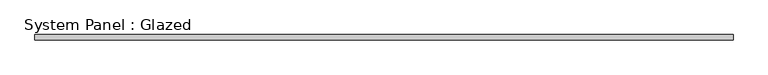
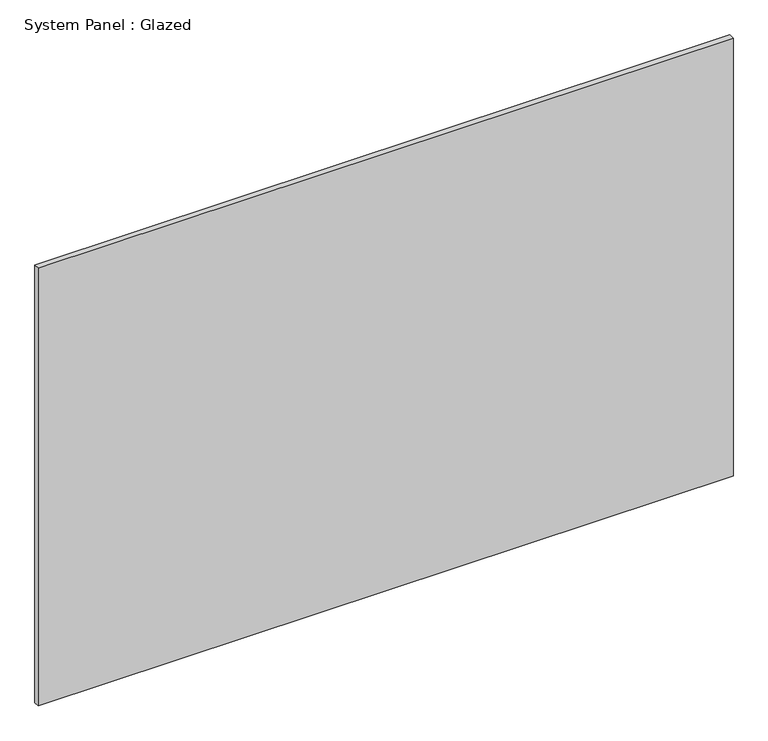
"""IFC4 building model written with IfcOpenShell, lengths in millimetres: plate geometry, System Panel : Glazed."""

from ifc_helpers import new_model, si_unit, origin, origin_with_axes, place, context, project, spatial, polyline, outline, extrude, source, transform, mapped, element, save


def system_panel_glazed_7ce5a3c2(model_context):
    return source(origin(), model_context, "Body", "SweptSolid", [
        extrude(outline(polyline([(1600.2, 19.05), (-1600.2, 19.05), (-1600.2, 44.45), (1600.2, 44.45), (1600.2, 19.05)])), origin_with_axes(), (0.0, 0.0, 1.0), 2133.6),
    ])


if __name__ == "__main__":
    model = new_model("IFC4")
    model_context = context("Model", 3, world=origin())
    ifc_project = project(units=[si_unit("LENGTHUNIT", "METRE", prefix="MILLI")], contexts=[model_context])
    site = spatial("IfcSite", under=ifc_project)
    building = spatial("IfcBuilding", under=site)
    placement = place(None, origin())
    system_panel_glazed_shape = system_panel_glazed_7ce5a3c2(model_context)
    element("IfcPlate", 1, ObjectType="System Panel : Glazed", at=placement, inside=building, context=model_context, shape_type="MappedRepresentation", body=[
        mapped(system_panel_glazed_shape, transform((0.0, 0.0, 0.0), x_axis=(1.0, 0.0, 0.0), y_axis=(0.0, 1.0, 0.0), z_axis=(0.0, 0.0, 1.0))),
    ])
    save(model, "model.ifc")

# Revit data of these elements
# Type "System Panel : Glazed"
#   Construction Type Id = "GSP4R"
#   Analytic Construction = "1/8 in Pilkington single glazing"
#   Visual Light Transmittance = 0.9
#   Solar Heat Gain Coefficient = 0.86
#   Heat Transfer Coefficient (U) = 1.18115 BTU/(h·ft²·°F)
# Element 1 (IfcPlate, "System Panel : Glazed")
#   Materials on its faces: "Glass"
# Materials
#   "Glass": class "Glass", colour RGB 0 128 192, transparency 0.75, Description = "Soda Lime Glass", Cost = 0
